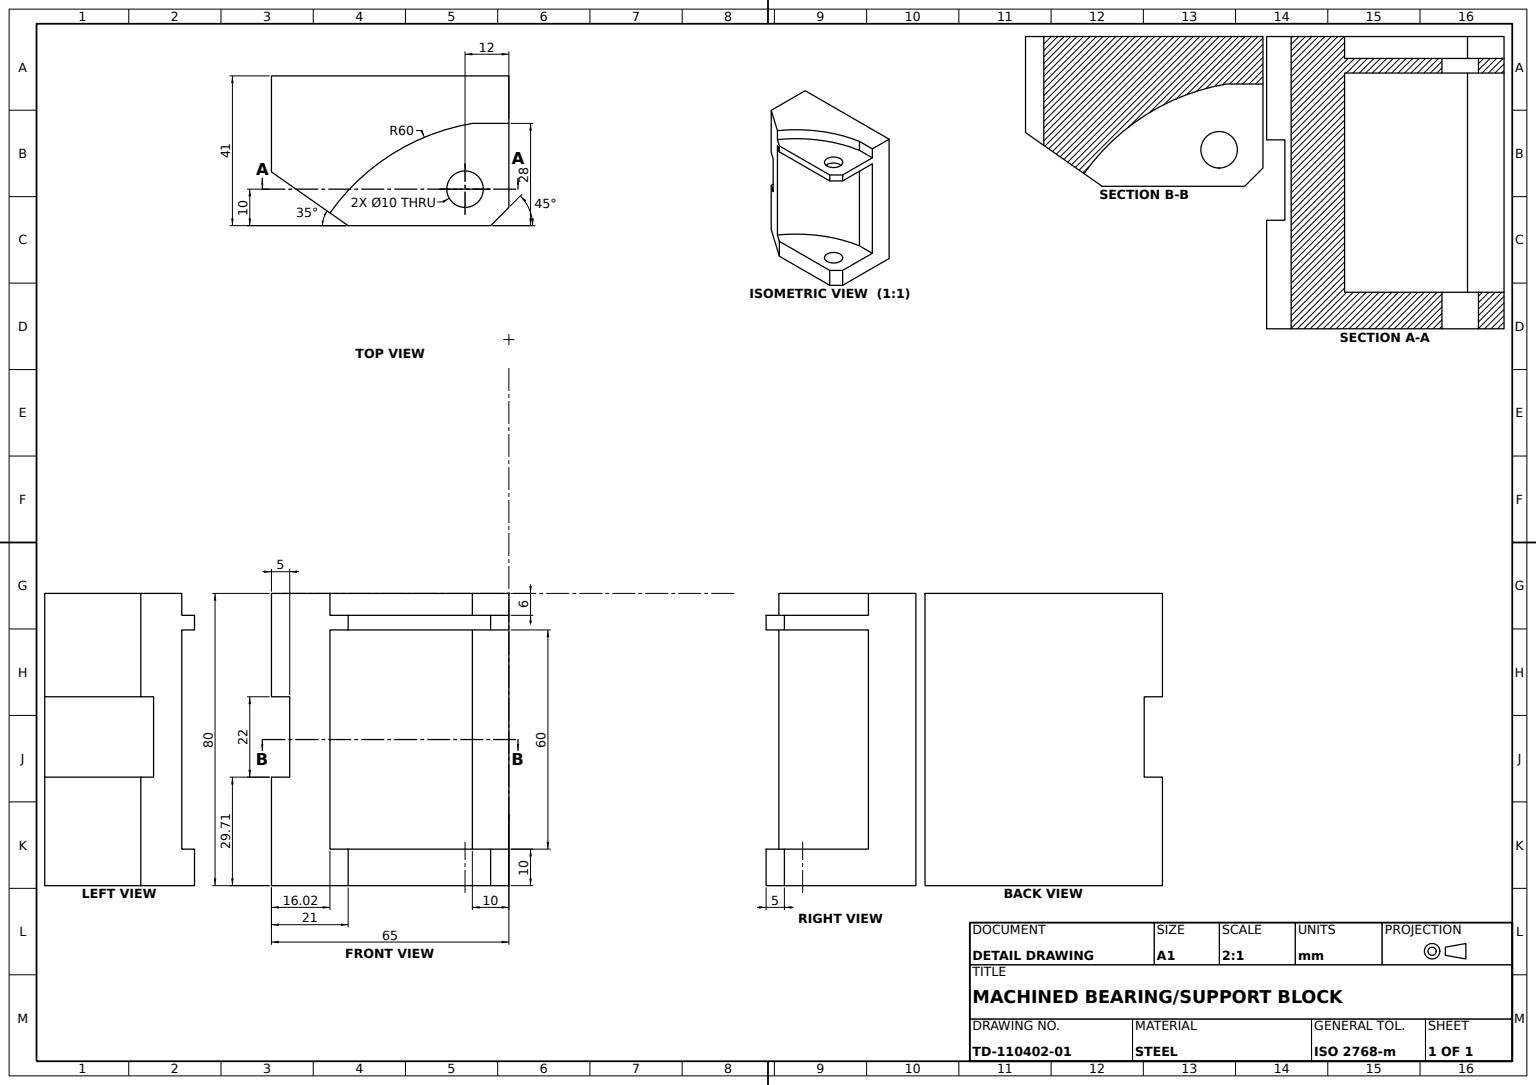
from build123d import *

# Parameters (mm, degrees)
BASE_BLOCK_DEPTH      = 40
SIDE_SLOT_DEPTH       = 56.466205928
SIDE_SLOT_DEPTH_BACK  = 56.466205928
SIDE_SLOT_SKETCH_W    = 5
SIDE_SLOT_SKETCH_H    = 22
TOP_STEP_POCKET_DEPTH = 6
ARC_RELIEF_CUT_DEPTH  = 30
THROUGH_HOLE_SKETCH_R = 5
THROUGH_HOLE_DEPTH    = 110


with BuildPart() as part:
    # Base Block Profile Sketch → Base Block (new, symmetric)
    with BuildSketch(Plane(origin=(0, 0, 0), x_dir=(1, 0, 0), z_dir=(0, 1, 0))):
        Polygon((11.5, 20.5), (32.5, 5.795641698), (32.5, -20.5), (-32.5, -20.5), (-32.5, 15.5), (-27.5, 20.5), align=None)
    extrude(amount=BASE_BLOCK_DEPTH, both=True)

    # Side Slot Sketch → Side Slot (cut, two sides: drawn at the far end of the back side and taken through both)
    with BuildSketch(Plane.XY.offset(-SIDE_SLOT_DEPTH_BACK)):
        with Locations((30, 0.707540159)):
            Rectangle(SIDE_SLOT_SKETCH_W, SIDE_SLOT_SKETCH_H)
    extrude(amount=SIDE_SLOT_DEPTH + SIDE_SLOT_DEPTH_BACK, mode=Mode.SUBTRACT)

    # Top Step Pocket Sketch → Top Step Pocket (cut)
    with BuildSketch(Plane(origin=(0, 40, 0), x_dir=(1, 0, 0), z_dir=(0, 1, 0))):
        with BuildLine():
            Line((16.483327146, 17.010636767), (11.5, 20.5))
            Line((11.5, 20.5), (-27.5, 20.5))
            Line((-27.5, 20.5), (-32.5, 15.5))
            Line((-32.5, 15.5), (-32.5, -7.5))
            Line((-32.5, -7.5), (-22.5, -7.5))
            ThreePointArc((-22.5, -7.5), (-0.563327522, 0.866615575), (16.483327146, 17.010636767))
        make_face()
    extrude(amount=-TOP_STEP_POCKET_DEPTH, mode=Mode.SUBTRACT)

    # Arc Relief Sketch → Arc Relief Cut (cut, symmetric)
    with BuildSketch(Plane(origin=(0, 0, 0), x_dir=(1, 0, 0), z_dir=(0, 1, 0))):
        with BuildLine():
            Line((-27.5, 20.5), (-32.5, 15.5))
            Line((-32.5, 15.5), (-32.5, -7.5))
            Line((-32.5, -7.5), (-22.5, -7.5))
            ThreePointArc((-22.5, -7.5), (-0.563327522, 0.866615575), (16.483327146, 17.010636767))
            Line((16.483327146, 17.010636767), (11.5, 20.5))
            Line((11.5, 20.5), (-27.5, 20.5))
        make_face()
    extrude(amount=ARC_RELIEF_CUT_DEPTH, both=True, mode=Mode.SUBTRACT)

    # Through Hole Sketch → Through Hole (cut)
    with BuildSketch(Plane(origin=(0, 34, 0), x_dir=(1, 0, 0), z_dir=(0, 1, 0))):
        with Locations(Location((-20.5, 10.5, 0), (0, 0, 270))):
            Circle(THROUGH_HOLE_SKETCH_R)
    extrude(amount=-THROUGH_HOLE_DEPTH, mode=Mode.SUBTRACT)


solid = part.part
